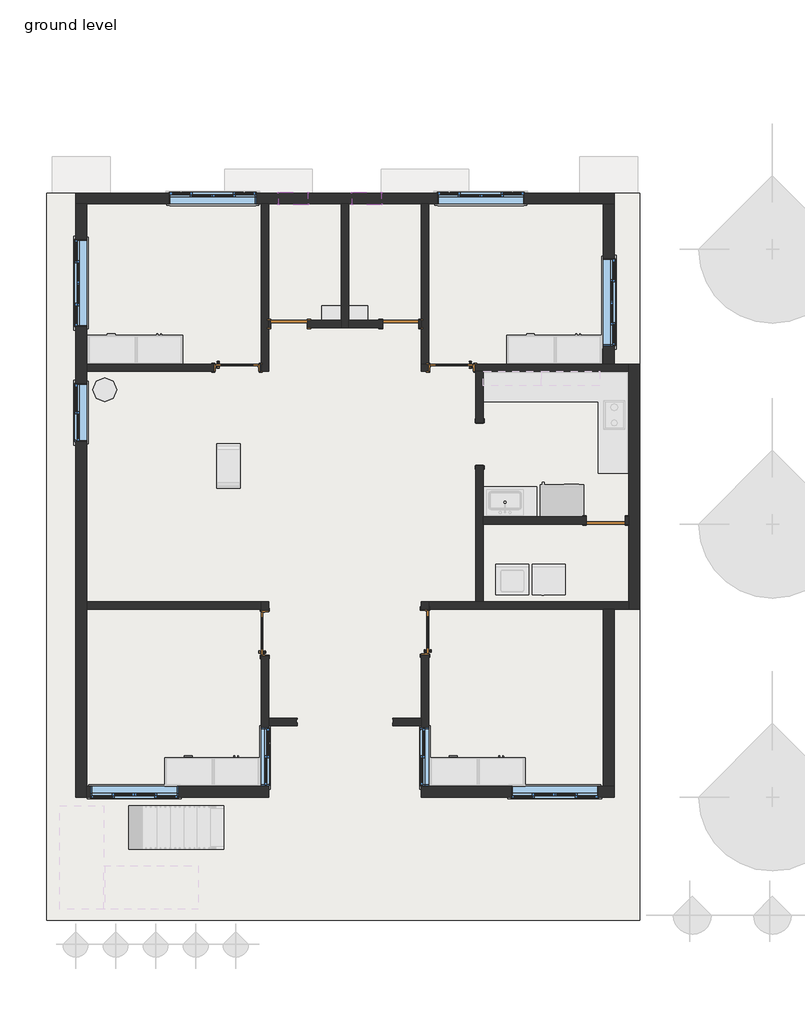
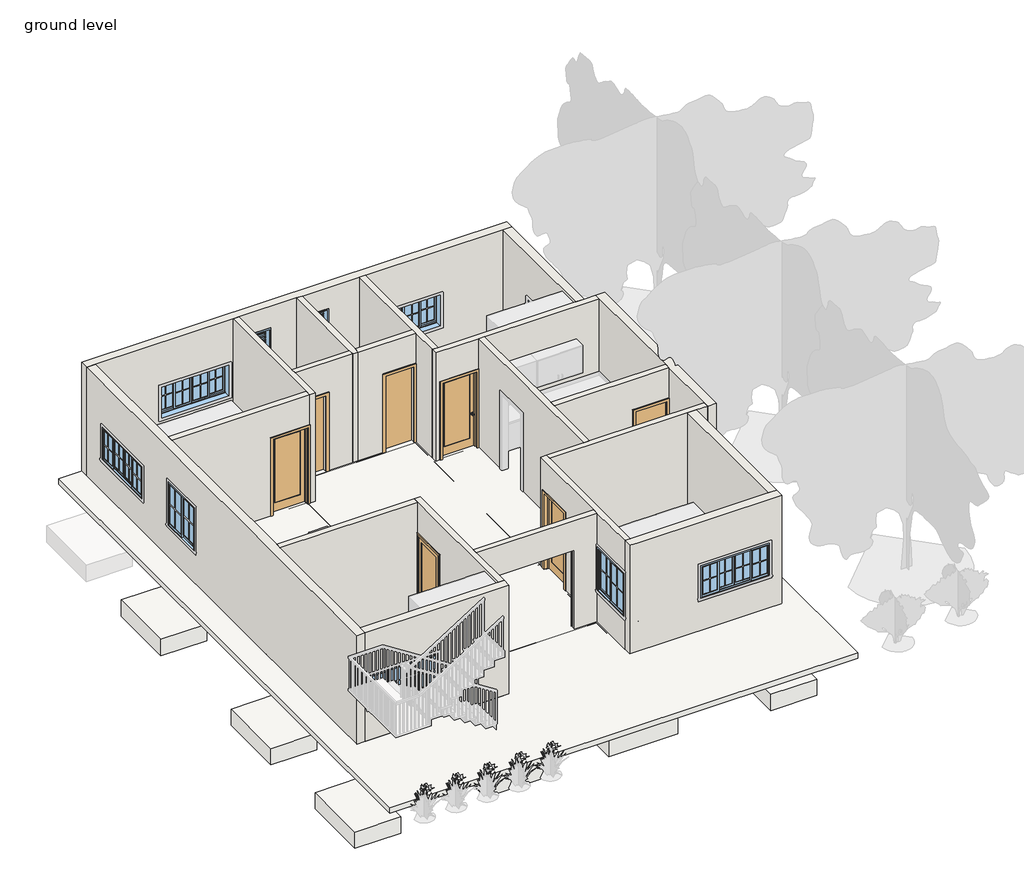
# One storey, part 1 of 4: 21 walls, 11 windows, 10 slabs, 7 beams, 7 doors.
"""IFC4 building model written with IfcOpenShell, lengths in millimetres."""

from ifc_helpers import new_model, si_unit, frame, origin, place, context, project, spatial, polyline, outline, extrude, faceted_brep, transform, mapped, element, save
from components import door_010cc4d9, door_5a860750, door_e2b13fe9, door_a9addea7, door_bb092f7c, window_f2d8fef0, window_c1e3dfc0, window_49fe3060, window_58cce754

model = new_model("IFC4")

# Units and contexts
model_context = context("Model", 3, world=origin())
ifc_project = project(units=[si_unit("LENGTHUNIT", "METRE", prefix="MILLI")], contexts=[model_context])

# Site, building, storey
site = spatial("IfcSite", under=ifc_project)
building = spatial("IfcBuilding", under=site)
storey = spatial("IfcBuildingStorey", under=building, Name="ground level", Elevation=609.6)

# Beams
placement = place(None, origin())
element("IfcBeam", 1, ObjectType="Concrete-Rectangular Beam", at=placement, inside=storey, context=model_context, shape_type="SweptSolid", body=[
    extrude(outline(polyline([(-1593.2124084, 1316.1961804), (-1364.6124084, 1316.1961804), (-1364.6124084, -2163.6038196), (-1593.2124084, -2163.6038196), (-1593.2124084, 1316.1961804)])), frame((0.0, 0.0, 304.8), z_axis=(0.0, 0.0, 1.0), x_axis=(1.0, 0.0, 0.0)), (0.0, 0.0, 1.0), 304.8),
])
element("IfcBeam", 2, ObjectType="Concrete-Rectangular Beam", at=placement, inside=storey, context=model_context, shape_type="Brep", body=[
    faceted_brep([(-1593.2124084, -2430.3038196, 609.6), (-1593.2124084, -2201.7038196, 609.6), (-5212.7124084, -2201.7038196, 609.6), (-5441.3124084, -2201.7038196, 609.6), (-5441.3124084, -2239.8038196, 609.6), (-5174.6124084, -2239.8038196, 609.6), (-5174.6124084, -2430.3038196, 609.6), (-1593.2124084, -2201.7038196, 304.8), (-5212.7124084, -2201.7038196, 304.8), (-5441.3124084, -2201.7038196, 304.8), (-1593.2124084, -2430.3038196, 304.8), (-5174.6124084, -2430.3038196, 304.8), (-5174.6124084, -2239.8038196, 304.8), (-5441.3124084, -2239.8038196, 304.8)], [[[0, 1, 2, 3, 4, 5, 6]], [[1, 7, 8, 9, 3, 2]], [[7, 10, 11, 12, 13, 9, 8]], [[6, 11, 10, 0]], [[0, 10, 7, 1]], [[12, 5, 4, 13]], [[5, 12, 11, 6]], [[3, 9, 13, 4]]]),
])
element("IfcBeam", 3, ObjectType="Concrete-Rectangular Beam", at=placement, inside=storey, context=model_context, shape_type="Brep", body=[
    faceted_brep([(-8756.0124084, -2468.4038196, 609.6), (-8756.0124084, -2239.8038196, 609.6), (-8794.1124084, -2239.8038196, 609.6), (-12413.6124084, -2239.8038196, 609.6), (-12413.6124084, -2468.4038196, 609.6), (-8756.0124084, -2239.8038196, 304.8), (-8794.1124084, -2239.8038196, 304.8), (-12413.6124084, -2239.8038196, 304.8), (-8756.0124084, -2468.4038196, 304.8), (-12413.6124084, -2468.4038196, 304.8)], [[[0, 1, 2, 3, 4]], [[1, 5, 6, 7, 3, 2]], [[5, 8, 9, 7, 6]], [[8, 0, 4, 9]], [[1, 0, 8, 5]], [[4, 3, 7, 9]]]),
])
element("IfcBeam", 4, ObjectType="Concrete-Rectangular Beam", at=placement, inside=storey, context=model_context, shape_type="SweptSolid", body=[
    extrude(outline(polyline([(-12642.2124084, 9875.9961804), (-12413.6124084, 9875.9961804), (-12413.6124084, 6751.7961804), (-12642.2124084, 6751.7961804), (-12642.2124084, 9875.9961804)])), frame((0.0, 0.0, 304.8), z_axis=(0.0, 0.0, 1.0), x_axis=(1.0, 0.0, 0.0)), (0.0, 0.0, 1.0), 304.8),
    extrude(outline(polyline([(-12413.6124084, -2163.6038196), (-12642.2124084, -2163.6038196), (-12642.2124084, 1392.3961804), (-12413.6124084, 1392.3961804), (-12413.6124084, -2163.6038196)])), frame((0.0, 0.0, 304.8), z_axis=(0.0, 0.0, 1.0), x_axis=(1.0, 0.0, 0.0)), (0.0, 0.0, 1.0), 304.8),
    extrude(outline(polyline([(-12413.6124084, 1697.1961804), (-12642.2124084, 1697.1961804), (-12642.2124084, 6446.9961804), (-12413.6124084, 6446.9961804), (-12413.6124084, 1697.1961804)])), frame((0.0, 0.0, 304.8), z_axis=(0.0, 0.0, 1.0), x_axis=(1.0, 0.0, 0.0)), (0.0, 0.0, 1.0), 304.8),
])
element("IfcBeam", 5, ObjectType="Concrete-Rectangular Beam", at=placement, inside=storey, context=model_context, shape_type="Brep", body=[
    faceted_brep([(-843.9124084, 1659.0961804, 609.6), (-843.9124084, 1430.4961804, 609.6), (-843.9124084, 1430.4961804, 304.8), (-843.9124084, 1659.0961804, 304.8), (-5098.4124084, 1659.0961804, 609.6), (-5098.4124084, 1468.5961804, 609.6), (-5403.2124084, 1468.5961804, 609.6), (-5403.2124084, 1659.0961804, 609.6), (-5441.3124084, 1659.0961804, 609.6), (-8565.5124084, 1659.0961804, 609.6), (-8603.6124084, 1659.0961804, 609.6), (-8603.6124084, 1468.5961804, 609.6), (-8908.4124084, 1468.5961804, 609.6), (-8908.4124084, 1659.0961804, 609.6), (-12413.6124084, 1659.0961804, 609.6), (-12413.6124084, 1430.4961804, 609.6), (-8794.1124084, 1430.4961804, 609.6), (-8565.5124084, 1430.4961804, 609.6), (-5441.3124084, 1430.4961804, 609.6), (-5212.7124084, 1430.4961804, 609.6), (-1593.2124084, 1430.4961804, 609.6), (-1593.2124084, 1620.9961804, 609.6), (-1364.6124084, 1620.9961804, 609.6), (-1364.6124084, 1430.4961804, 609.6), (-1364.6124084, 1430.4961804, 304.8), (-1364.6124084, 1620.9961804, 304.8), (-1593.2124084, 1620.9961804, 304.8), (-1593.2124084, 1430.4961804, 304.8), (-5212.7124084, 1430.4961804, 304.8), (-5441.3124084, 1430.4961804, 304.8), (-8565.5124084, 1430.4961804, 304.8), (-8794.1124084, 1430.4961804, 304.8), (-12413.6124084, 1430.4961804, 304.8), (-12413.6124084, 1659.0961804, 304.8), (-8908.4124084, 1659.0961804, 304.8), (-8908.4124084, 1468.5961804, 304.8), (-8603.6124084, 1468.5961804, 304.8), (-8603.6124084, 1659.0961804, 304.8), (-8565.5124084, 1659.0961804, 304.8), (-5441.3124084, 1659.0961804, 304.8), (-5403.2124084, 1659.0961804, 304.8), (-5403.2124084, 1468.5961804, 304.8), (-5098.4124084, 1468.5961804, 304.8), (-5098.4124084, 1659.0961804, 304.8)], [[[0, 1, 2, 3]], [[1, 0, 4, 5, 6, 7, 8, 9, 10, 11, 12, 13, 14, 15, 16, 17, 18, 19, 20, 21, 22, 23]], [[2, 1, 23, 24]], [[3, 2, 24, 25, 26, 27, 28, 29, 30, 31, 32, 33, 34, 35, 36, 37, 38, 39, 40, 41, 42, 43]], [[0, 3, 43, 4]], [[15, 14, 33, 32]], [[22, 25, 24, 23]], [[26, 21, 20, 27]], [[21, 26, 25, 22]], [[36, 11, 10, 37]], [[11, 36, 35, 12]], [[12, 35, 34, 13]], [[42, 5, 4, 43]], [[5, 42, 41, 6]], [[6, 41, 40, 7]], [[15, 32, 31, 30, 29, 28, 27, 20, 19, 18, 17, 16]], [[33, 14, 13, 34]], [[37, 10, 9, 8, 7, 40, 39, 38]]]),
])
element("IfcBeam", 6, ObjectType="Concrete-Rectangular Beam", at=placement, inside=storey, context=model_context, shape_type="Brep", body=[
    faceted_brep([(-8794.1124084, -2239.8038196, 609.6), (-8756.0124084, -2239.8038196, 609.6), (-8565.5124084, -2239.8038196, 609.6), (-8565.5124084, -1007.9038196, 609.6), (-8565.5124084, -779.3038196, 609.6), (-8565.5124084, 1430.4961804, 609.6), (-8794.1124084, 1430.4961804, 609.6), (-8794.1124084, -2239.8038196, 304.8), (-8794.1124084, 1430.4961804, 304.8), (-8565.5124084, -2239.8038196, 304.8), (-8756.0124084, -2239.8038196, 304.8), (-8565.5124084, 1430.4961804, 304.8), (-8565.5124084, -779.3038196, 304.8), (-8565.5124084, -1007.9038196, 304.8)], [[[0, 1, 2, 3, 4, 5, 6]], [[7, 0, 6, 8]], [[9, 10, 7, 8, 11, 12, 13]], [[2, 9, 13, 12, 11, 5, 4, 3]], [[2, 1, 0, 7, 10, 9]], [[6, 5, 11, 8]]]),
    faceted_brep([(-8794.1124084, 9914.0961804, 609.6), (-8565.5124084, 9914.0961804, 609.6), (-8565.5124084, 9914.0961804, 304.8), (-8794.1124084, 9914.0961804, 304.8), (-8756.0124084, 6751.7961804, 304.8), (-8756.0124084, 6751.7961804, 609.6), (-8756.0124084, 6713.6961804, 609.6), (-8756.0124084, 6713.6961804, 304.8), (-8565.5124084, 6751.7961804, 304.8), (-8565.5124084, 6751.7961804, 609.6), (-8794.1124084, 6713.6961804, 609.6), (-8794.1124084, 6713.6961804, 304.8), (-8565.5124084, 7323.2961804, 609.6), (-8565.5124084, 7551.8961804, 609.6), (-8565.5124084, 7551.8961804, 304.8), (-8565.5124084, 7323.2961804, 304.8)], [[[0, 1, 2, 3]], [[4, 5, 6, 7]], [[5, 4, 8, 9]], [[6, 10, 11, 7]], [[1, 0, 10, 6, 5, 9, 12, 13]], [[3, 2, 14, 15, 8, 4, 7, 11]], [[2, 1, 13, 12, 9, 8, 15, 14]], [[0, 3, 11, 10]]]),
    faceted_brep([(-8756.0124084, 6446.9961804, 304.8), (-8756.0124084, 6446.9961804, 609.6), (-8565.5124084, 6446.9961804, 609.6), (-8565.5124084, 6446.9961804, 304.8), (-8603.6124084, 1697.1961804, 304.8), (-8603.6124084, 1697.1961804, 609.6), (-8794.1124084, 1697.1961804, 609.6), (-8794.1124084, 1697.1961804, 304.8), (-8603.6124084, 1659.0961804, 304.8), (-8603.6124084, 1659.0961804, 609.6), (-8794.1124084, 6485.0961804, 609.6), (-8756.0124084, 6485.0961804, 609.6), (-8756.0124084, 6485.0961804, 304.8), (-8794.1124084, 6485.0961804, 304.8), (-8565.5124084, 1659.0961804, 609.6), (-8565.5124084, 1659.0961804, 304.8)], [[[0, 1, 2, 3]], [[4, 5, 6, 7]], [[5, 4, 8, 9]], [[10, 11, 12, 13]], [[14, 9, 8, 15]], [[7, 6, 10, 13]], [[1, 0, 12, 11]], [[11, 10, 6, 5, 9, 14, 2, 1]], [[13, 12, 0, 3, 15, 8, 4, 7]], [[3, 2, 14, 15]]]),
])
element("IfcBeam", 7, ObjectType="Concrete-Rectangular Beam", at=placement, inside=storey, context=model_context, shape_type="SweptSolid", body=[
    extrude(outline(polyline([(-5441.3124084, -779.3038196), (-5441.3124084, -1007.9038196), (-8565.5124084, -1007.9038196), (-8565.5124084, -779.3038196), (-5441.3124084, -779.3038196)])), frame((0.0, 0.0, 304.8), z_axis=(0.0, 0.0, 1.0), x_axis=(1.0, 0.0, 0.0)), (0.0, 0.0, 1.0), 304.8),
])

# Doors
door_shape = door_010cc4d9(model_context)
element("IfcDoor", 8, ObjectType="Door-Interior-Single-1_Panel-Wood : 36\" x 84\"", at=placement, inside=storey, context=model_context, shape_type="MappedRepresentation", body=[
    mapped(door_shape, transform((-9264.0124084, 6526.3711804, 609.6), x_axis=(1.0, 0.0, 0.0), y_axis=(0.0, 1.0, 0.0), z_axis=(0.0, 0.0, 1.0))),
])
element("IfcDoor", 9, ObjectType="Door-Interior-Single-1_Panel-Wood : 36\" x 84\"", at=placement, inside=storey, context=model_context, shape_type="MappedRepresentation", body=[
    mapped(door_shape, transform((-8682.9874084, 960.5961804, 609.6), x_axis=(0.0, 1.0, 0.0), y_axis=(-1.0, 0.0, 0.0), z_axis=(0.0, 0.0, 1.0))),
])
door_2_shape = door_5a860750(model_context)
element("IfcDoor", 10, ObjectType="Door-Interior-Single-1_Panel-Wood : 36\" x 84\"", at=placement, inside=storey, context=model_context, shape_type="MappedRepresentation", body=[
    mapped(door_2_shape, transform((-4768.2124084, 6526.3711804, 609.6), x_axis=(-1.0, 0.0, 0.0), y_axis=(0.0, -1.0, 0.0), z_axis=(0.0, 0.0, 1.0))),
])
element("IfcDoor", 11, ObjectType="Door-Interior-Single-1_Panel-Wood : 36\" x 84\"", at=placement, inside=storey, context=model_context, shape_type="MappedRepresentation", body=[
    mapped(door_2_shape, transform((-5323.8374084, 985.9961804, 609.6), x_axis=(0.0, 1.0, 0.0), y_axis=(-1.0, 0.0, 0.0), z_axis=(0.0, 0.0, 1.0))),
])
door_3_shape = door_e2b13fe9(model_context)
element("IfcDoor", 12, ObjectType="Single-Flush : 30\" x 84\"", at=placement, inside=storey, context=model_context, shape_type="MappedRepresentation", body=[
    mapped(door_3_shape, transform((-8171.8124084, 7437.5961804, 609.6), x_axis=(-1.0, 0.0, 0.0), y_axis=(0.0, -1.0, 0.0), z_axis=(0.0, 0.0, 1.0))),
])
door_4_shape = door_a9addea7(model_context)
element("IfcDoor", 13, ObjectType="Single-Flush : 30\" x 84\"", at=placement, inside=storey, context=model_context, shape_type="MappedRepresentation", body=[
    mapped(door_4_shape, transform((-5835.0124084, 7437.5961804, 609.6), x_axis=(1.0, 0.0, 0.0), y_axis=(0.0, 1.0, 0.0), z_axis=(0.0, 0.0, 1.0))),
])
door_5_shape = door_bb092f7c(model_context)
element("IfcDoor", 14, ObjectType="Single-Flush : 32\" x 84\"", at=placement, inside=storey, context=model_context, shape_type="MappedRepresentation", body=[
    mapped(door_5_shape, transform((-1542.4124084, 3322.7961804, 609.6), x_axis=(1.0, 0.0, 0.0), y_axis=(0.0, 1.0, 0.0), z_axis=(0.0, 0.0, 1.0))),
])

# Slabs
element("IfcSlab", 15, ObjectType="Footing-Rectangular : 72\" x 48\" x 18\"", at=placement, inside=storey, context=model_context, shape_type="SweptSolid", body=[
    extrude(outline(polyline([(-869.3124084, -1401.6038196), (-869.3124084, -3230.4038196), (-2088.5124084, -3230.4038196), (-2088.5124084, -1401.6038196), (-869.3124084, -1401.6038196)])), frame((0.0, 0.0, -1676.4), z_axis=(0.0, 0.0, 1.0), x_axis=(1.0, 0.0, 0.0)), (0.0, 0.0, 1.0), 457.2),
])
element("IfcSlab", 16, ObjectType="Footing-Rectangular : 72\" x 48\" x 18\"", at=placement, inside=storey, context=model_context, shape_type="SweptSolid", body=[
    extrude(outline(polyline([(-6241.4124084, -1744.5038196), (-4412.6124084, -1744.5038196), (-4412.6124084, -2963.7038196), (-6241.4124084, -2963.7038196), (-6241.4124084, -1744.5038196)])), frame((0.0, 0.0, -1676.4), z_axis=(0.0, 0.0, 1.0), x_axis=(1.0, 0.0, 0.0)), (0.0, 0.0, 1.0), 457.2),
])
element("IfcSlab", 17, ObjectType="Footing-Rectangular : 72\" x 48\" x 18\"", at=placement, inside=storey, context=model_context, shape_type="SweptSolid", body=[
    extrude(outline(polyline([(-9518.0124084, -1744.5038196), (-7689.2124084, -1744.5038196), (-7689.2124084, -2963.7038196), (-9518.0124084, -2963.7038196), (-9518.0124084, -1744.5038196)])), frame((0.0, 0.0, -1676.4), z_axis=(0.0, 0.0, 1.0), x_axis=(1.0, 0.0, 0.0)), (0.0, 0.0, 1.0), 457.2),
])
element("IfcSlab", 18, ObjectType="Footing-Rectangular : 72\" x 48\" x 18\"", at=placement, inside=storey, context=model_context, shape_type="SweptSolid", body=[
    extrude(outline(polyline([(-13137.5124084, -3230.4038196), (-13137.5124084, -1401.6038196), (-11918.3124084, -1401.6038196), (-11918.3124084, -3230.4038196), (-13137.5124084, -3230.4038196)])), frame((0.0, 0.0, -1676.4), z_axis=(0.0, 0.0, 1.0), x_axis=(1.0, 0.0, 0.0)), (0.0, 0.0, 1.0), 457.2),
])
element("IfcSlab", 19, ObjectType="Footing-Rectangular : 72\" x 48\" x 18\"", at=placement, inside=storey, context=model_context, shape_type="SweptSolid", body=[
    extrude(outline(polyline([(-11918.3124084, 2459.1961804), (-11918.3124084, 630.3961804), (-13137.5124084, 630.3961804), (-13137.5124084, 2459.1961804), (-11918.3124084, 2459.1961804)])), frame((0.0, 0.0, -1676.4), z_axis=(0.0, 0.0, 1.0), x_axis=(1.0, 0.0, 0.0)), (0.0, 0.0, 1.0), 457.2),
])
element("IfcSlab", 20, ObjectType="Footing-Rectangular : 72\" x 48\" x 18\"", at=placement, inside=storey, context=model_context, shape_type="SweptSolid", body=[
    extrude(outline(polyline([(-11918.3124084, 7513.7961804), (-11918.3124084, 5684.9961804), (-13137.5124084, 5684.9961804), (-13137.5124084, 7513.7961804), (-11918.3124084, 7513.7961804)])), frame((0.0, 0.0, -1676.4), z_axis=(0.0, 0.0, 1.0), x_axis=(1.0, 0.0, 0.0)), (0.0, 0.0, 1.0), 457.2),
])
element("IfcSlab", 21, ObjectType="Footing-Rectangular : 72\" x 48\" x 18\"", at=placement, inside=storey, context=model_context, shape_type="SweptSolid", body=[
    extrude(outline(polyline([(-8032.1124084, 7513.7961804), (-8032.1124084, 5684.9961804), (-9251.3124084, 5684.9961804), (-9251.3124084, 7513.7961804), (-8032.1124084, 7513.7961804)])), frame((0.0, 0.0, -1676.4), z_axis=(0.0, 0.0, 1.0), x_axis=(1.0, 0.0, 0.0)), (0.0, 0.0, 1.0), 457.2),
])
element("IfcSlab", 22, ObjectType="Footing-Rectangular : 72\" x 48\" x 18\"", at=placement, inside=storey, context=model_context, shape_type="SweptSolid", body=[
    extrude(outline(polyline([(-9670.4124084, 2192.4961804), (-7841.6124084, 2192.4961804), (-7841.6124084, 973.2961804), (-9670.4124084, 973.2961804), (-9670.4124084, 2192.4961804)])), frame((0.0, 0.0, -1676.4), z_axis=(0.0, 0.0, 1.0), x_axis=(1.0, 0.0, 0.0)), (0.0, 0.0, 1.0), 457.2),
])
element("IfcSlab", 23, ObjectType="Footing-Rectangular : 72\" x 48\" x 18\"", at=placement, inside=storey, context=model_context, shape_type="SweptSolid", body=[
    extrude(outline(polyline([(-6165.2124084, 2192.4961804), (-4336.4124084, 2192.4961804), (-4336.4124084, 973.2961804), (-6165.2124084, 973.2961804), (-6165.2124084, 2192.4961804)])), frame((0.0, 0.0, -1676.4), z_axis=(0.0, 0.0, 1.0), x_axis=(1.0, 0.0, 0.0)), (0.0, 0.0, 1.0), 457.2),
])
element("IfcSlab", 24, ObjectType="Generic - 6\"", at=placement, inside=storey, context=model_context, shape_type="SweptSolid", body=[
    extrude(outline(polyline([(-831.2124084, 10180.7961804), (-831.2124084, -5046.5038196), (-13251.8124084, -5046.5038196), (-13251.8124084, 10180.7961804), (-831.2124084, 10180.7961804)])), frame((0.0, 0.0, 457.2), z_axis=(0.0, 0.0, 1.0), x_axis=(1.0, 0.0, 0.0)), (0.0, 0.0, 1.0), 152.4),
])

# Walls
element("IfcWall", 25, ObjectType="Generic - 6\"", at=placement, inside=storey, context=model_context, shape_type="Brep", body=[
    faceted_brep([(-8756.0124084, 9952.1961804, 609.6), (-8756.0124084, 6599.3961804, 609.6), (-8756.0124084, 6446.9961804, 609.6), (-8756.0124084, 6446.9961804, 3657.6), (-8756.0124084, 6599.3961804, 3657.6), (-8756.0124084, 9952.1961804, 3657.6), (-8603.6124084, 9952.1961804, 609.6), (-8603.6124084, 9952.1961804, 3657.6), (-8603.6124084, 7513.7961804, 3657.6), (-8603.6124084, 7361.3961804, 3657.6), (-8603.6124084, 6446.9961804, 3657.6), (-8603.6124084, 6446.9961804, 609.6), (-8603.6124084, 7361.3961804, 609.6), (-8603.6124084, 7513.7961804, 609.6)], [[[0, 1, 2, 3, 4, 5]], [[6, 7, 8, 9, 10, 11, 12, 13]], [[2, 1, 0, 6, 13, 12, 11]], [[0, 5, 7, 6]], [[3, 2, 11, 10]], [[5, 4, 3, 10, 9, 8, 7]]]),
])
element("IfcWall", 26, ObjectType="Generic - 6\"", at=placement, inside=storey, context=model_context, shape_type="SweptSolid", body=[
    extrude(outline(polyline([(609.6, -8756.0124084), (3657.6, -8756.0124084), (3657.6, -12413.6124084), (609.6, -12413.6124084), (609.6, -9746.6124084), (2768.6, -9746.6124084), (2768.6, -8781.4124084), (609.6, -8781.4124084), (609.6, -8756.0124084)])), frame((0.0, 6446.9961804, 0.0), z_axis=(0.0, 1.0, 0.0), x_axis=(0.0, 0.0, 1.0)), (0.0, 0.0, 1.0), 152.4),
])
element("IfcWall", 27, ObjectType="Generic - 6\"", at=placement, inside=storey, context=model_context, shape_type="Brep", body=[
    faceted_brep([(-7079.6124084, 9952.1961804, 609.6), (-7079.6124084, 7513.7961804, 609.6), (-7079.6124084, 7361.3961804, 609.6), (-7079.6124084, 7361.3961804, 3657.6), (-7079.6124084, 7513.7961804, 3657.6), (-7079.6124084, 9952.1961804, 3657.6), (-6927.2124084, 9952.1961804, 609.6), (-6927.2124084, 9952.1961804, 3657.6), (-6927.2124084, 7513.7961804, 3657.6), (-6927.2124084, 7361.3961804, 3657.6), (-6927.2124084, 7361.3961804, 609.6), (-6927.2124084, 7513.7961804, 609.6)], [[[0, 1, 2, 3, 4, 5]], [[6, 7, 8, 9, 10, 11]], [[2, 1, 0, 6, 11, 10]], [[0, 5, 7, 6]], [[3, 2, 10, 9]], [[5, 4, 3, 9, 8, 7]]]),
])
element("IfcWall", 28, ObjectType="Generic - 6\"", at=placement, inside=storey, context=model_context, shape_type="SweptSolid", body=[
    extrude(outline(polyline([(609.6, -7079.6124084), (3657.6, -7079.6124084), (3657.6, -8603.6124084), (609.6, -8603.6124084), (609.6, -8552.8124084), (2743.2, -8552.8124084), (2743.2, -7790.8124084), (609.6, -7790.8124084), (609.6, -7079.6124084)])), frame((0.0, 7361.3961804, 0.0), z_axis=(0.0, 1.0, 0.0), x_axis=(0.0, 0.0, 1.0)), (0.0, 0.0, 1.0), 152.4),
])
element("IfcWall", 29, ObjectType="Generic - 6\"", at=placement, inside=storey, context=model_context, shape_type="SweptSolid", body=[
    extrude(outline(polyline([(3657.6, -6927.2124084), (609.6, -6927.2124084), (609.6, -6216.0124084), (2743.2, -6216.0124084), (2743.2, -5454.0124084), (609.6, -5454.0124084), (609.6, -5403.2124084), (3657.6, -5403.2124084), (3657.6, -6927.2124084)])), frame((0.0, 7361.3961804, 0.0), z_axis=(0.0, 1.0, 0.0), x_axis=(0.0, 0.0, 1.0)), (0.0, 0.0, 1.0), 152.4),
])
element("IfcWall", 30, ObjectType="Generic - 6\"", at=placement, inside=storey, context=model_context, shape_type="Brep", body=[
    faceted_brep([(-5250.8124084, 6599.3961804, 609.6), (-5250.8124084, 9952.1961804, 609.6), (-5250.8124084, 9952.1961804, 3657.6), (-5250.8124084, 6599.3961804, 3657.6), (-5403.2124084, 6599.3961804, 609.6), (-5403.2124084, 6599.3961804, 3657.6), (-5403.2124084, 7361.3961804, 3657.6), (-5403.2124084, 7513.7961804, 3657.6), (-5403.2124084, 9952.1961804, 3657.6), (-5403.2124084, 9952.1961804, 609.6), (-5403.2124084, 7513.7961804, 609.6), (-5403.2124084, 7361.3961804, 609.6)], [[[0, 1, 2, 3]], [[4, 5, 6, 7, 8, 9, 10, 11]], [[1, 0, 4, 11, 10, 9]], [[2, 1, 9, 8]], [[0, 3, 5, 4]], [[3, 2, 8, 7, 6, 5]]]),
])
element("IfcWall", 31, ObjectType="Generic - 6\"", at=placement, inside=storey, context=model_context, shape_type="Brep", body=[
    faceted_brep([(-5403.2124084, 6599.3961804, 609.6), (-5403.2124084, 6599.3961804, 3657.6), (-5250.8124084, 6599.3961804, 3657.6), (-1593.2124084, 6599.3961804, 3657.6), (-1364.6124084, 6599.3961804, 3657.6), (-1059.8124084, 6599.3961804, 3657.6), (-1059.8124084, 6599.3961804, 609.6), (-1364.6124084, 6599.3961804, 609.6), (-1593.2124084, 6599.3961804, 609.6), (-4285.6124084, 6599.3961804, 609.6), (-4285.6124084, 6599.3961804, 2768.6), (-5250.8124084, 6599.3961804, 2768.6), (-5250.8124084, 6599.3961804, 609.6), (-1059.8124084, 6446.9961804, 3657.6), (-4107.8124084, 6446.9961804, 3657.6), (-4260.2124084, 6446.9961804, 3657.6), (-5403.2124084, 6446.9961804, 3657.6), (-5403.2124084, 6446.9961804, 609.6), (-5250.8124084, 6446.9961804, 609.6), (-5250.8124084, 6446.9961804, 2768.6), (-4285.6124084, 6446.9961804, 2768.6), (-4285.6124084, 6446.9961804, 609.6), (-4260.2124084, 6446.9961804, 609.6), (-4107.8124084, 6446.9961804, 609.6), (-1059.8124084, 6446.9961804, 609.6)], [[[0, 1, 2, 3, 4, 5, 6, 7, 8, 9, 10, 11, 12]], [[13, 14, 15, 16, 17, 18, 19, 20, 21, 22, 23, 24]], [[17, 0, 12, 18]], [[6, 24, 23, 22, 21, 9, 8, 7]], [[1, 0, 17, 16]], [[6, 5, 13, 24]], [[11, 19, 18, 12]], [[19, 11, 10, 20]], [[20, 10, 9, 21]], [[16, 15, 14, 13, 5, 4, 3, 2, 1]]]),
])
element("IfcWall", 32, ObjectType="Generic - 6\"", at=placement, inside=storey, context=model_context, shape_type="SweptSolid", body=[
    extrude(outline(polyline([(-8756.0124084, 1468.5961804), (-12413.6124084, 1468.5961804), (-12413.6124084, 1620.9961804), (-8756.0124084, 1620.9961804), (-8756.0124084, 1468.5961804)])), frame((0.0, 0.0, 609.6), z_axis=(0.0, 0.0, 1.0), x_axis=(1.0, 0.0, 0.0)), (0.0, 0.0, 1.0), 3048.0),
])
element("IfcWall", 33, ObjectType="Generic - 6\"", at=placement, inside=storey, context=model_context, shape_type="Brep", body=[
    faceted_brep([(-5403.2124084, 1620.9961804, 3657.6), (-5403.2124084, 1620.9961804, 609.6), (-5403.2124084, 1468.5961804, 609.6), (-5403.2124084, 1468.5961804, 2768.6), (-5403.2124084, 503.3961804, 2768.6), (-5403.2124084, 503.3961804, 609.6), (-5403.2124084, -817.4038196, 609.6), (-5403.2124084, -969.8038196, 609.6), (-5403.2124084, -2239.8038196, 609.6), (-5403.2124084, -2239.8038196, 3657.6), (-5403.2124084, -969.8038196, 3657.6), (-5403.2124084, -817.4038196, 3657.6), (-5403.2124084, -1014.2538196, 1524.0), (-5403.2124084, -1014.2538196, 2743.2), (-5403.2124084, -2233.4538196, 2743.2), (-5403.2124084, -2233.4538196, 1524.0), (-5250.8124084, 1620.9961804, 609.6), (-5250.8124084, 1620.9961804, 3657.6), (-5250.8124084, 1468.5961804, 3657.6), (-5250.8124084, -2239.8038196, 3657.6), (-5250.8124084, -2239.8038196, 609.6), (-5250.8124084, 503.3961804, 609.6), (-5250.8124084, 503.3961804, 2768.6), (-5250.8124084, 1468.5961804, 2768.6), (-5250.8124084, 1468.5961804, 609.6), (-5250.8124084, -1014.2538196, 2743.2), (-5250.8124084, -1014.2538196, 1524.0), (-5250.8124084, -2233.4538196, 1524.0), (-5250.8124084, -2233.4538196, 2743.2)], [[[0, 1, 2, 3, 4, 5, 6, 7, 8, 9, 10, 11], [12, 13, 14, 15]], [[16, 17, 18, 19, 20, 21, 22, 23, 24], [25, 26, 27, 28]], [[1, 16, 24, 2]], [[8, 7, 6, 5, 21, 20]], [[1, 0, 17, 16]], [[23, 3, 2, 24]], [[3, 23, 22, 4]], [[4, 22, 21, 5]], [[25, 13, 12, 26]], [[26, 12, 15, 27]], [[27, 15, 14, 28]], [[13, 25, 28, 14]], [[0, 11, 10, 9, 19, 18, 17]], [[9, 8, 20, 19]]]),
])
element("IfcWall", 34, ObjectType="Generic - 6\"", at=placement, inside=storey, context=model_context, shape_type="Brep", body=[
    faceted_brep([(-8756.0124084, 1620.9961804, 609.6), (-8756.0124084, 1468.5961804, 609.6), (-8756.0124084, 1443.1961804, 609.6), (-8756.0124084, 1443.1961804, 2768.6), (-8756.0124084, 477.9961804, 2768.6), (-8756.0124084, 477.9961804, 609.6), (-8756.0124084, -2239.8038196, 609.6), (-8756.0124084, -2239.8038196, 3657.6), (-8756.0124084, 1468.5961804, 3657.6), (-8756.0124084, 1620.9961804, 3657.6), (-8756.0124084, -2233.4538196, 2743.2), (-8756.0124084, -2233.4538196, 1524.0), (-8756.0124084, -1014.2538196, 1524.0), (-8756.0124084, -1014.2538196, 2743.2), (-8603.6124084, 1443.1961804, 609.6), (-8603.6124084, 1620.9961804, 609.6), (-8603.6124084, 1620.9961804, 3657.6), (-8603.6124084, -817.4038196, 3657.6), (-8603.6124084, -969.8038196, 3657.6), (-8603.6124084, -2239.8038196, 3657.6), (-8603.6124084, -2239.8038196, 609.6), (-8603.6124084, -969.8038196, 609.6), (-8603.6124084, -817.4038196, 609.6), (-8603.6124084, 477.9961804, 609.6), (-8603.6124084, 477.9961804, 2768.6), (-8603.6124084, 1443.1961804, 2768.6), (-8603.6124084, -2233.4538196, 1524.0), (-8603.6124084, -2233.4538196, 2743.2), (-8603.6124084, -1014.2538196, 2743.2), (-8603.6124084, -1014.2538196, 1524.0)], [[[0, 1, 2, 3, 4, 5, 6, 7, 8, 9], [10, 11, 12, 13]], [[14, 15, 16, 17, 18, 19, 20, 21, 22, 23, 24, 25], [26, 27, 28, 29]], [[6, 5, 23, 22, 21, 20]], [[2, 1, 0, 15, 14]], [[25, 3, 2, 14]], [[3, 25, 24, 4]], [[4, 24, 23, 5]], [[0, 9, 16, 15]], [[10, 27, 26, 11]], [[11, 26, 29, 12]], [[12, 29, 28, 13]], [[27, 10, 13, 28]], [[9, 8, 7, 19, 18, 17, 16]], [[7, 6, 20, 19]]]),
])
element("IfcWall", 35, ObjectType="Generic - 6\"", at=placement, inside=storey, context=model_context, shape_type="Brep", body=[
    faceted_brep([(-4260.2124084, 6446.9961804, 3657.6), (-4260.2124084, 6446.9961804, 609.6), (-4260.2124084, 5380.1961804, 609.6), (-4260.2124084, 5380.1961804, 2743.2), (-4260.2124084, 4465.7961804, 2743.2), (-4260.2124084, 4465.7961804, 609.6), (-4260.2124084, 1620.9961804, 609.6), (-4260.2124084, 1620.9961804, 3657.6), (-4107.8124084, 6446.9961804, 609.6), (-4107.8124084, 6446.9961804, 3657.6), (-4107.8124084, 3398.9961804, 3657.6), (-4107.8124084, 3246.5961804, 3657.6), (-4107.8124084, 1620.9961804, 3657.6), (-4107.8124084, 1620.9961804, 609.6), (-4107.8124084, 3246.5961804, 609.6), (-4107.8124084, 3398.9961804, 609.6), (-4107.8124084, 4465.7961804, 609.6), (-4107.8124084, 4465.7961804, 2743.2), (-4107.8124084, 5380.1961804, 2743.2), (-4107.8124084, 5380.1961804, 609.6)], [[[0, 1, 2, 3, 4, 5, 6, 7]], [[8, 9, 10, 11, 12, 13, 14, 15, 16, 17, 18, 19]], [[1, 8, 19, 2]], [[13, 6, 5, 16, 15, 14]], [[1, 0, 9, 8]], [[7, 6, 13, 12]], [[4, 17, 16, 5]], [[18, 3, 2, 19]], [[17, 4, 3, 18]], [[0, 7, 12, 11, 10, 9]]]),
])
element("IfcWall", 36, ObjectType="Generic - 6\"", at=placement, inside=storey, context=model_context, shape_type="SweptSolid", body=[
    extrude(outline(polyline([(3657.6, -4107.8124084), (609.6, -4107.8124084), (609.6, -1948.8124084), (2743.2, -1948.8124084), (2743.2, -1136.0124084), (609.6, -1136.0124084), (609.6, -1059.8124084), (3657.6, -1059.8124084), (3657.6, -4107.8124084)])), frame((0.0, 3246.5961804, 0.0), z_axis=(0.0, 1.0, 0.0), x_axis=(0.0, 0.0, 1.0)), (0.0, 0.0, 1.0), 152.4),
])
element("IfcWall", 37, ObjectType="Generic - 6\"", at=placement, inside=storey, context=model_context, shape_type="Brep", body=[
    faceted_brep([(-5250.8124084, 1468.5961804, 609.6), (-1593.2124084, 1468.5961804, 609.6), (-1364.6124084, 1468.5961804, 609.6), (-1059.8124084, 1468.5961804, 609.6), (-1059.8124084, 1468.5961804, 3657.6), (-1364.6124084, 1468.5961804, 3657.6), (-1593.2124084, 1468.5961804, 3657.6), (-5250.8124084, 1468.5961804, 3657.6), (-5250.8124084, 1620.9961804, 609.6), (-5250.8124084, 1620.9961804, 3657.6), (-4260.2124084, 1620.9961804, 3657.6), (-4107.8124084, 1620.9961804, 3657.6), (-1059.8124084, 1620.9961804, 3657.6), (-1059.8124084, 1620.9961804, 609.6), (-4107.8124084, 1620.9961804, 609.6), (-4260.2124084, 1620.9961804, 609.6)], [[[0, 1, 2, 3, 4, 5, 6, 7]], [[8, 9, 10, 11, 12, 13, 14, 15]], [[3, 2, 1, 0, 8, 15, 14, 13]], [[4, 3, 13, 12]], [[0, 7, 9, 8]], [[7, 6, 5, 4, 12, 11, 10, 9]]]),
])
element("IfcWall", 38, ObjectType="Generic - 6\"", at=placement, inside=storey, context=model_context, shape_type="Brep", body=[
    faceted_brep([(-5403.2124084, -969.8038196, 609.6), (-5403.2124084, -969.8038196, 3657.6), (-8603.6124084, -969.8038196, 3657.6), (-8603.6124084, -969.8038196, 609.6), (-8003.4124084, -969.8038196, 609.6), (-8003.4124084, -969.8038196, 2818.6), (-6003.4124084, -969.8038196, 2818.6), (-6003.4124084, -969.8038196, 609.6), (-5403.2124084, -817.4038196, 3657.6), (-5403.2124084, -817.4038196, 609.6), (-6003.4124084, -817.4038196, 609.6), (-6003.4124084, -817.4038196, 2818.6), (-8003.4124084, -817.4038196, 2818.6), (-8003.4124084, -817.4038196, 609.6), (-8603.6124084, -817.4038196, 609.6), (-8603.6124084, -817.4038196, 3657.6), (-8003.4124084, -837.4038196, 609.6), (-8018.4124084, -837.4038196, 609.6), (-8018.4124084, -907.4038196, 609.6), (-8003.4124084, -907.4038196, 609.6), (-6003.4124084, -907.4038196, 609.6), (-5988.4124084, -907.4038196, 609.6), (-5988.4124084, -837.4038196, 609.6), (-6003.4124084, -837.4038196, 609.6), (-6003.4124084, -837.4038196, 2818.6), (-8003.4124084, -837.4038196, 2818.6), (-8003.4124084, -907.4038196, 2818.6), (-6003.4124084, -907.4038196, 2818.6), (-8018.4124084, -907.4038196, 2833.6), (-5988.4124084, -907.4038196, 2833.6), (-5988.4124084, -837.4038196, 2833.6), (-8018.4124084, -837.4038196, 2833.6)], [[[0, 1, 2, 3, 4, 5, 6, 7]], [[8, 9, 10, 11, 12, 13, 14, 15]], [[3, 14, 13, 16, 17, 18, 19, 4]], [[9, 0, 7, 20, 21, 22, 23, 10]], [[1, 0, 9, 8]], [[3, 2, 15, 14]], [[24, 25, 12, 11]], [[26, 27, 6, 5]], [[19, 26, 5, 4]], [[27, 20, 7, 6]], [[27, 26, 19, 18, 28, 29, 21, 20]], [[21, 29, 30, 22]], [[25, 24, 23, 22, 30, 31, 17, 16]], [[23, 24, 11, 10]], [[25, 16, 13, 12]], [[28, 18, 17, 31]], [[29, 28, 31, 30]], [[2, 1, 8, 15]]]),
])
element("IfcWall", 39, ObjectType="Generic - 9\"", at=placement, inside=storey, context=model_context, shape_type="Brep", body=[
    faceted_brep([(-12642.2124084, 9952.1961804, 609.6), (-12413.6124084, 9952.1961804, 609.6), (-8756.0124084, 9952.1961804, 609.6), (-8603.6124084, 9952.1961804, 609.6), (-7079.6124084, 9952.1961804, 609.6), (-6927.2124084, 9952.1961804, 609.6), (-5403.2124084, 9952.1961804, 609.6), (-5250.8124084, 9952.1961804, 609.6), (-1593.2124084, 9952.1961804, 609.6), (-1364.6124084, 9952.1961804, 609.6), (-1364.6124084, 9952.1961804, 3657.6), (-1593.2124084, 9952.1961804, 3657.6), (-5250.8124084, 9952.1961804, 3657.6), (-5403.2124084, 9952.1961804, 3657.6), (-6927.2124084, 9952.1961804, 3657.6), (-7079.6124084, 9952.1961804, 3657.6), (-8603.6124084, 9952.1961804, 3657.6), (-8756.0124084, 9952.1961804, 3657.6), (-12413.6124084, 9952.1961804, 3657.6), (-12642.2124084, 9952.1961804, 3657.6), (-3244.2124084, 9952.1961804, 2438.4), (-3244.2124084, 9952.1961804, 1524.0), (-5073.0124084, 9952.1961804, 1524.0), (-5073.0124084, 9952.1961804, 2438.4), (-8857.6124084, 9952.1961804, 2438.4), (-8857.6124084, 9952.1961804, 1524.0), (-10686.4124084, 9952.1961804, 1524.0), (-10686.4124084, 9952.1961804, 2438.4), (-8387.7124084, 9952.1961804, 2438.4), (-8387.7124084, 9952.1961804, 3048.0), (-7778.1124084, 9952.1961804, 3048.0), (-7778.1124084, 9952.1961804, 2438.4), (-6851.0124084, 9952.1961804, 2438.4), (-6851.0124084, 9952.1961804, 3048.0), (-6241.4124084, 9952.1961804, 3048.0), (-6241.4124084, 9952.1961804, 2438.4), (-1364.6124084, 10180.7961804, 609.6), (-12642.2124084, 10180.7961804, 609.6), (-12642.2124084, 10180.7961804, 3657.6), (-1364.6124084, 10180.7961804, 3657.6), (-3244.2124084, 10180.7961804, 1524.0), (-3244.2124084, 10180.7961804, 2438.4), (-5073.0124084, 10180.7961804, 2438.4), (-5073.0124084, 10180.7961804, 1524.0), (-8857.6124084, 10180.7961804, 1524.0), (-8857.6124084, 10180.7961804, 2438.4), (-10686.4124084, 10180.7961804, 2438.4), (-10686.4124084, 10180.7961804, 1524.0), (-8387.7124084, 10180.7961804, 3048.0), (-8387.7124084, 10180.7961804, 2438.4), (-7778.1124084, 10180.7961804, 2438.4), (-7778.1124084, 10180.7961804, 3048.0), (-6851.0124084, 10180.7961804, 3048.0), (-6851.0124084, 10180.7961804, 2438.4), (-6241.4124084, 10180.7961804, 2438.4), (-6241.4124084, 10180.7961804, 3048.0)], [[[0, 1, 2, 3, 4, 5, 6, 7, 8, 9, 10, 11, 12, 13, 14, 15, 16, 17, 18, 19], [20, 21, 22, 23], [24, 25, 26, 27], [28, 29, 30, 31], [32, 33, 34, 35]], [[36, 37, 38, 39], [40, 41, 42, 43], [44, 45, 46, 47], [48, 49, 50, 51], [52, 53, 54, 55]], [[9, 8, 7, 6, 5, 4, 3, 2, 1, 0, 37, 36]], [[0, 19, 38, 37]], [[10, 9, 36, 39]], [[20, 41, 40, 21]], [[21, 40, 43, 22]], [[22, 43, 42, 23]], [[41, 20, 23, 42]], [[24, 45, 44, 25]], [[25, 44, 47, 26]], [[46, 27, 26, 47]], [[45, 24, 27, 46]], [[49, 48, 29, 28]], [[50, 49, 28, 31]], [[51, 50, 31, 30]], [[48, 51, 30, 29]], [[53, 52, 33, 32]], [[54, 53, 32, 35]], [[55, 54, 35, 34]], [[52, 55, 34, 33]], [[19, 18, 17, 16, 15, 14, 13, 12, 11, 10, 39, 38]]]),
])
element("IfcWall", 40, ObjectType="Generic - 9\"", at=placement, inside=storey, context=model_context, shape_type="Brep", body=[
    faceted_brep([(-12642.2124084, 9952.1961804, 609.6), (-12642.2124084, -2468.4038196, 609.6), (-12642.2124084, -2468.4038196, 3657.6), (-12642.2124084, 9952.1961804, 3657.6), (-12642.2124084, 4973.7961804, 2743.2), (-12642.2124084, 4973.7961804, 1524.0), (-12642.2124084, 6192.9961804, 1524.0), (-12642.2124084, 6192.9961804, 2743.2), (-12642.2124084, 9209.2461804, 1524.0), (-12642.2124084, 9209.2461804, 2438.4), (-12642.2124084, 7380.4461804, 2438.4), (-12642.2124084, 7380.4461804, 1524.0), (-12413.6124084, -2468.4038196, 609.6), (-12413.6124084, -2239.8038196, 609.6), (-12413.6124084, 1468.5961804, 609.6), (-12413.6124084, 1620.9961804, 609.6), (-12413.6124084, 6446.9961804, 609.6), (-12413.6124084, 6599.3961804, 609.6), (-12413.6124084, 9952.1961804, 609.6), (-12413.6124084, 9952.1961804, 3657.6), (-12413.6124084, 6599.3961804, 3657.6), (-12413.6124084, 6446.9961804, 3657.6), (-12413.6124084, 1620.9961804, 3657.6), (-12413.6124084, 1468.5961804, 3657.6), (-12413.6124084, -2239.8038196, 3657.6), (-12413.6124084, -2468.4038196, 3657.6), (-12413.6124084, 4973.7961804, 1524.0), (-12413.6124084, 4973.7961804, 2743.2), (-12413.6124084, 6192.9961804, 2743.2), (-12413.6124084, 6192.9961804, 1524.0), (-12413.6124084, 9209.2461804, 2438.4), (-12413.6124084, 9209.2461804, 1524.0), (-12413.6124084, 7380.4461804, 1524.0), (-12413.6124084, 7380.4461804, 2438.4)], [[[0, 1, 2, 3], [4, 5, 6, 7], [8, 9, 10, 11]], [[12, 13, 14, 15, 16, 17, 18, 19, 20, 21, 22, 23, 24, 25], [26, 27, 28, 29], [30, 31, 32, 33]], [[1, 0, 18, 17, 16, 15, 14, 13, 12]], [[0, 3, 19, 18]], [[2, 1, 12, 25]], [[4, 27, 26, 5]], [[5, 26, 29, 6]], [[6, 29, 28, 7]], [[30, 9, 8, 31]], [[31, 8, 11, 32]], [[10, 33, 32, 11]], [[9, 30, 33, 10]], [[27, 4, 7, 28]], [[3, 2, 25, 24, 23, 22, 21, 20, 19]]]),
])
element("IfcWall", 41, ObjectType="Generic - 9\"", at=placement, inside=storey, context=model_context, shape_type="SweptSolid", body=[
    extrude(outline(polyline([(9952.1961804, 609.6), (6599.3961804, 609.6), (6599.3961804, 3657.6), (9952.1961804, 3657.6), (9952.1961804, 609.6)]), holes=[polyline([(6980.3961804, 2438.4), (6980.3961804, 1524.0), (8809.1961804, 1524.0), (8809.1961804, 2438.4), (6980.3961804, 2438.4)])]), frame((-1593.2124084, 0.0, 0.0), z_axis=(1.0, 0.0, 0.0), x_axis=(0.0, 1.0, 0.0)), (0.0, 0.0, 1.0), 228.6),
])
element("IfcWall", 42, ObjectType="Generic - 9\"", at=placement, inside=storey, context=model_context, shape_type="Brep", body=[
    faceted_brep([(-12413.6124084, -2468.4038196, 609.6), (-8603.6124084, -2468.4038196, 609.6), (-8603.6124084, -2468.4038196, 3657.6), (-12413.6124084, -2468.4038196, 3657.6), (-12324.7124084, -2468.4038196, 1524.0), (-12324.7124084, -2468.4038196, 2438.4), (-10495.9124084, -2468.4038196, 2438.4), (-10495.9124084, -2468.4038196, 1524.0), (-8603.6124084, -2239.8038196, 609.6), (-8756.0124084, -2239.8038196, 609.6), (-12413.6124084, -2239.8038196, 609.6), (-12413.6124084, -2239.8038196, 3657.6), (-8756.0124084, -2239.8038196, 3657.6), (-8603.6124084, -2239.8038196, 3657.6), (-12324.7124084, -2239.8038196, 2438.4), (-12324.7124084, -2239.8038196, 1524.0), (-10495.9124084, -2239.8038196, 1524.0), (-10495.9124084, -2239.8038196, 2438.4)], [[[0, 1, 2, 3], [4, 5, 6, 7]], [[8, 9, 10, 11, 12, 13], [14, 15, 16, 17]], [[1, 0, 10, 9, 8]], [[0, 3, 11, 10]], [[14, 5, 4, 15]], [[15, 4, 7, 16]], [[16, 7, 6, 17]], [[5, 14, 17, 6]], [[3, 2, 13, 12, 11]], [[2, 1, 8, 13]]]),
])
element("IfcWall", 43, ObjectType="Generic - 9\"", at=placement, inside=storey, context=model_context, shape_type="SweptSolid", body=[
    extrude(outline(polyline([(-1593.2124084, -2239.8038196), (-1593.2124084, 1468.5961804), (-1364.6124084, 1468.5961804), (-1364.6124084, -2239.8038196), (-1593.2124084, -2239.8038196)])), frame((0.0, 0.0, 609.6), z_axis=(0.0, 0.0, 1.0), x_axis=(1.0, 0.0, 0.0)), (0.0, 0.0, 1.0), 3048.0),
])
element("IfcWall", 44, ObjectType="Generic - 9\"", at=placement, inside=storey, context=model_context, shape_type="Brep", body=[
    faceted_brep([(-1059.8124084, 6599.3961804, 609.6), (-1059.8124084, 6446.9961804, 609.6), (-1059.8124084, 3398.9961804, 609.6), (-1059.8124084, 3246.5961804, 609.6), (-1059.8124084, 1620.9961804, 609.6), (-1059.8124084, 1468.5961804, 609.6), (-1059.8124084, 1468.5961804, 3657.6), (-1059.8124084, 1620.9961804, 3657.6), (-1059.8124084, 3246.5961804, 3657.6), (-1059.8124084, 3398.9961804, 3657.6), (-1059.8124084, 6446.9961804, 3657.6), (-1059.8124084, 6599.3961804, 3657.6), (-831.2124084, 6599.3961804, 609.6), (-831.2124084, 6599.3961804, 3657.6), (-831.2124084, 1468.5961804, 3657.6), (-831.2124084, 1468.5961804, 609.6)], [[[0, 1, 2, 3, 4, 5, 6, 7, 8, 9, 10, 11]], [[12, 13, 14, 15]], [[5, 4, 3, 2, 1, 0, 12, 15]], [[0, 11, 13, 12]], [[6, 5, 15, 14]], [[11, 10, 9, 8, 7, 6, 14, 13]]]),
])
element("IfcWall", 45, ObjectType="Generic - 9\"", at=placement, inside=storey, context=model_context, shape_type="Brep", body=[
    faceted_brep([(-5403.2124084, -2468.4038196, 609.6), (-1364.6124084, -2468.4038196, 609.6), (-1364.6124084, -2468.4038196, 3657.6), (-5174.6124084, -2468.4038196, 3657.6), (-5403.2124084, -2468.4038196, 3657.6), (-3523.6124084, -2468.4038196, 1524.0), (-3523.6124084, -2468.4038196, 2438.4), (-1694.8124084, -2468.4038196, 2438.4), (-1694.8124084, -2468.4038196, 1524.0), (-1364.6124084, -2239.8038196, 609.6), (-1593.2124084, -2239.8038196, 609.6), (-5250.8124084, -2239.8038196, 609.6), (-5403.2124084, -2239.8038196, 609.6), (-5403.2124084, -2239.8038196, 3657.6), (-5250.8124084, -2239.8038196, 3657.6), (-1593.2124084, -2239.8038196, 3657.6), (-1364.6124084, -2239.8038196, 3657.6), (-3523.6124084, -2239.8038196, 2438.4), (-3523.6124084, -2239.8038196, 1524.0), (-1694.8124084, -2239.8038196, 1524.0), (-1694.8124084, -2239.8038196, 2438.4)], [[[0, 1, 2, 3, 4], [5, 6, 7, 8]], [[9, 10, 11, 12, 13, 14, 15, 16], [17, 18, 19, 20]], [[1, 0, 12, 11, 10, 9]], [[2, 1, 9, 16]], [[17, 6, 5, 18]], [[18, 5, 8, 19]], [[19, 8, 7, 20]], [[6, 17, 20, 7]], [[16, 15, 14, 13, 4, 3, 2]], [[0, 4, 13, 12]]]),
])

# Windows
window_shape = window_f2d8fef0(model_context)
element("IfcWindow", 46, ObjectType="Window-Louvers : 24\" x 24\"", at=placement, inside=storey, context=model_context, shape_type="MappedRepresentation", body=[
    mapped(window_shape, transform((-8082.9124084, 10072.8461804, 1524.0), x_axis=(1.0, 0.0, 0.0), y_axis=(0.0, 1.0, 0.0), z_axis=(0.0, 0.0, 1.0))),
])
element("IfcWindow", 47, ObjectType="Window-Louvers : 24\" x 24\"", at=placement, inside=storey, context=model_context, shape_type="MappedRepresentation", body=[
    mapped(window_shape, transform((-6546.2124084, 10072.8461804, 1524.0), x_axis=(1.0, 0.0, 0.0), y_axis=(0.0, 1.0, 0.0), z_axis=(0.0, 0.0, 1.0))),
])
window_2_shape = window_c1e3dfc0(model_context)
element("IfcWindow", 48, ObjectType="Window-Sliding-Double : 48\" x 48\"", at=placement, inside=storey, context=model_context, shape_type="MappedRepresentation", body=[
    mapped(window_2_shape, transform((-12531.7224084, 5583.3961804, 609.6), x_axis=(0.0, -1.0, 0.0), y_axis=(1.0, 0.0, 0.0), z_axis=(0.0, 0.0, 1.0))),
])
window_3_shape = window_49fe3060(model_context)
element("IfcWindow", 49, ObjectType="Window-Sliding-Double : 48\" x 48\"", at=placement, inside=storey, context=model_context, shape_type="MappedRepresentation", body=[
    mapped(window_3_shape, transform((-8676.0024084, -1623.8538196, 609.6), x_axis=(0.0, -1.0, 0.0), y_axis=(1.0, 0.0, 0.0), z_axis=(0.0, 0.0, 1.0))),
])
element("IfcWindow", 50, ObjectType="Window-Sliding-Double : 48\" x 48\"", at=placement, inside=storey, context=model_context, shape_type="MappedRepresentation", body=[
    mapped(window_3_shape, transform((-5330.8224084, -1623.8538196, 609.6), x_axis=(0.0, 1.0, 0.0), y_axis=(-1.0, 0.0, 0.0), z_axis=(0.0, 0.0, 1.0))),
])
window_4_shape = window_58cce754(model_context)
element("IfcWindow", 51, ObjectType="Window-Sliding-Four : 72\" x 36\"", at=placement, inside=storey, context=model_context, shape_type="MappedRepresentation", body=[
    mapped(window_4_shape, transform((-9772.0124084, 10070.3061804, 609.6), x_axis=(1.0, 0.0, 0.0), y_axis=(0.0, 1.0, 0.0), z_axis=(0.0, 0.0, 1.0))),
])
element("IfcWindow", 52, ObjectType="Window-Sliding-Four : 72\" x 36\"", at=placement, inside=storey, context=model_context, shape_type="MappedRepresentation", body=[
    mapped(window_4_shape, transform((-12531.7224084, 8294.8461804, 609.6), x_axis=(0.0, 1.0, 0.0), y_axis=(-1.0, 0.0, 0.0), z_axis=(0.0, 0.0, 1.0))),
])
element("IfcWindow", 53, ObjectType="Window-Sliding-Four : 72\" x 36\"", at=placement, inside=storey, context=model_context, shape_type="MappedRepresentation", body=[
    mapped(window_4_shape, transform((-1475.1024084, 7894.7961804, 609.6), x_axis=(0.0, -1.0, 0.0), y_axis=(1.0, 0.0, 0.0), z_axis=(0.0, 0.0, 1.0))),
])
element("IfcWindow", 54, ObjectType="Window-Sliding-Four : 72\" x 36\"", at=placement, inside=storey, context=model_context, shape_type="MappedRepresentation", body=[
    mapped(window_4_shape, transform((-4158.6124084, 10070.3061804, 609.6), x_axis=(1.0, 0.0, 0.0), y_axis=(0.0, 1.0, 0.0), z_axis=(0.0, 0.0, 1.0))),
])
element("IfcWindow", 55, ObjectType="Window-Sliding-Four : 72\" x 36\"", at=placement, inside=storey, context=model_context, shape_type="MappedRepresentation", body=[
    mapped(window_4_shape, transform((-2609.2124084, -2357.9138196, 609.6), x_axis=(-1.0, 0.0, 0.0), y_axis=(0.0, -1.0, 0.0), z_axis=(0.0, 0.0, 1.0))),
])
element("IfcWindow", 56, ObjectType="Window-Sliding-Four : 72\" x 36\"", at=placement, inside=storey, context=model_context, shape_type="MappedRepresentation", body=[
    mapped(window_4_shape, transform((-11410.3124084, -2357.9138196, 609.6), x_axis=(-1.0, 0.0, 0.0), y_axis=(0.0, -1.0, 0.0), z_axis=(0.0, 0.0, 1.0))),
])

save(model, "model.ifc")

# Revit data of these elements
# Type "Concrete-Rectangular Beam"
#   Assembly Code = "B10"
#   Length [instance default] = 5' - 0"
#   b = 0' - 9"
#   h = 1' - 0"
#   Structural Material [instance default] = Concrete, Cast-in-Place gray
# Type "Door-Interior-Single-1_Panel-Wood : 36\" x 84\""
#   Type Mark = "8"
#   Assembly Code = "C1020300"
#   Analytic Construction = "Wooden"
#   Top Rail = 0' - 4 11/16"
#   Thickness = 0' - 1 3/8"
#   Thermal Resistance (R) = 2.5876 (h·ft²·°F)/BTU
#   Swing Angle [instance default] = 90.00°
#   Stiles = 0' - 4 3/4"
#   Rough Width = 3' - 2"
#   Rough Height = 7' - 1"
#   Height = 7' - 0"
#   Width = 3' - 0"
#   Heat Transfer Coefficient (U) = 0.3865 BTU/(h·ft²·°F)
#   Bottom Rail = 0' - 9 1/8"
#   Trim Material = Cherry
#   Panel Material = Cherry
#   Frame Material = Cherry
#   Door Handle Material = Aluminum
#   Visual Light Transmittance = 0
#   Solar Heat Gain Coefficient = 0
#   Wall Closure = (empty or 0)
#   Function = (empty or 0)
# Type "Single-Flush : 30\" x 84\""
#   Type Mark = "4"
#   Construction Type Id = "MDOOR"
#   Assembly Code = "C1020"
#   Analytic Construction = "Metal"
#   Thickness = 0' - 2"
#   Heat Transfer Coefficient (U) = 0.651978 BTU/(h·ft²·°F)
#   Height = 7' - 0"
#   Trim Projection Ext = 0' - 1"
#   Trim Projection Int = 0' - 1"
#   Trim Width = 0' - 3"
#   Width = 2' - 6"
#   Define Thermal Properties by = 1
#   Define Thermal Properties by = 1
#   Door Material = Door - Panel
#   Frame Material = Door - Frame
#   Visual Light Transmittance = 0
#   Solar Heat Gain Coefficient = 0
#   Function = (empty or 0)
#   Wall Closure = (empty or 0)
# Type "Single-Flush : 32\" x 84\""
#   Type Mark = "3"
#   Construction Type Id = "MDOOR"
#   Assembly Code = "C1020"
#   Analytic Construction = "Metal"
#   Thickness = 0' - 2"
#   Heat Transfer Coefficient (U) = 0.651978 BTU/(h·ft²·°F)
#   Height = 7' - 0"
#   Trim Projection Ext = 0' - 1"
#   Trim Projection Int = 0' - 1"
#   Trim Width = 0' - 3"
#   Width = 2' - 8"
#   Define Thermal Properties by = 1
#   Define Thermal Properties by = 1
#   Door Material = Door - Panel
#   Frame Material = Door - Frame
#   Visual Light Transmittance = 0
#   Solar Heat Gain Coefficient = 0
#   Function = (empty or 0)
#   Wall Closure = (empty or 0)
# Type "Footing-Rectangular : 72\" x 48\" x 18\""
#   Assembly Code = "A1010100"
#   Width = 4' - 0"
#   Length = 6' - 0"
#   Foundation Thickness = 1' - 6"
#   Structural Material [instance default] = Concrete, Cast-in-Place gray
# Type "Generic - 6\""
#   Assembly Code = "B1010"
#   Function = 0
#   Layers, outside or top first: 0' - 6" no material (function 1)
# Type "Generic - 6\""
#   Assembly Code = "B2010"
#   Layers, outside or top first: 0' - 6" no material (function 1)
# Type "Generic - 9\""
#   Assembly Code = "B2010"
#   Layers, outside or top first: 0' - 9" no material (function 1)
# Type "Window-Louvers : 24\" x 24\""
#   Type Mark = "24"
#   Construction Type Id = "GSP4R"
#   Assembly Code = "B20"
#   Analytic Construction = "1/8 in Pilkington single glazing"
#   Visual Light Transmittance = 0.9
#   Thermal Resistance (R) = 1.53941 (h·ft²·°F)/BTU
#   Solar Heat Gain Coefficient = 0.78
#   Max Height = 1' - 11.74264"
#   Height = 2' - 0"
#   Heat Transfer Coefficient (U) = 0.6496 BTU/(h·ft²·°F)
#   Blade Width [instance default] = 1' - 10 1/2"
#   Blade Vertical Thickness = 0' - 0.35355"
#   Blade Thickness = 0' - 0 1/4"
#   Blade Spacing = 0' - 1 1/2"
#   Blade Height = 0' - 1.85355"
#   Blade Depth = 0' - 3"
#   Blade Angle = 45.00°
#   Default Sill Height = 3' - 0"
#   Trim Projection_Exterior = 0' - 0 1/2"
#   Trim Projection_Interior = 0' - 0 1/2"
#   Trim Width_Exterior = 0' - 1 1/2"
#   Trim Width_Interior = 0' - 1 1/2"
#   Width = 2' - 0"
#   Max Blade Count = 12
#   Define Thermal Properties by = 1
#   Blade Count = 12
#   Frame Material = Birch
#   Louver Material = Birch
#   Trim Exterior Material = Birch
#   Trim Interior Material = Birch
#   Wall Closure = (empty or 0)
# Type "Window-Sliding-Double : 48\" x 48\""
#   Type Mark = "23"
#   Fire Rating = "0.5h"
#   Assembly Code = "B2020100"
#   Analytic Construction = "Double glazing - domestic"
#   Window Inset [instance default] = 0' - 0"
#   Wall Thickness [instance default] = 0' - 6"
#   Visual Light Transmittance = 0.81
#   Thermal Resistance (R) = 1.8146 (h·ft²·°F)/BTU
#   Solar Heat Gain Coefficient = 0.76
#   Muntin Width = 1' - 8 5/8"
#   Muntin Height = 3' - 6 1/4"
#   Interior Wall Closure [instance default] = 0' - 2 3/4"
#   Heat Transfer Coefficient (U) = 0.5511 BTU/(h·ft²·°F)
#   Frame Extension [instance default] = 0' - 0 1/4"
#   Exterior Wall Closure [instance default] = 0' - 1 1/4"
#   Rough Width = 4' - 0 1/2"
#   Rough Height = 4' - 0 1/2"
#   Height = 4' - 0"
#   Extension Jamb [instance default] = 0' - 2 3/4"
#   Default Sill Height = 3' - 0"
#   Width = 4' - 0"
#   Interior Trim Visibility [instance default] = yes
#   Indicator Visibility [instance default] = yes
#   Exterior Trim Visibility [instance default] = yes
#   Muntin Visibility = yes
#   Extension Jamb Visibility [instance default] = yes
#   Muntin Pattern = Muntin Pattern_2x2 : Muntin Pattern_2x2
#   Interior Trim Material = Wood - Stained
#   Interior Trim = Trim-Window-Interior-Flat : Picture Frame
#   Interior Frame Material = Wood - Stained
#   Glass Panel Material = Glass
#   Exterior Trim Material = Clad - White
#   Exterior Trim = Trim-Window-Exterior-Flat : with Sill
#   Exterior Frame Material = Clad - White
#   Wall Closure = (empty or 0)
# Type "Window-Sliding-Four : 72\" x 36\""
#   Type Mark = "20"
#   Fire Rating = "0.5h"
#   Assembly Code = "B2020100"
#   Analytic Construction = "Double glazing - domestic"
#   Window Inset [instance default] = 0' - 0"
#   Wall Thickness [instance default] = 0' - 6"
#   Visual Light Transmittance = 0.81
#   Thermal Resistance (R) = 1.8146 (h·ft²·°F)/BTU
#   Solar Heat Gain Coefficient = 0.76
#   Interior Wall Closure [instance default] = 0' - 2 19/32"
#   Heat Transfer Coefficient (U) = 0.5511 BTU/(h·ft²·°F)
#   Frame Extension [instance default] = 0' - 0 1/4"
#   Exterior Wall Closure [instance default] = 0' - 1 1/4"
#   Rough Width = 6' - 0 1/2"
#   Rough Height = 3' - 0 1/2"
#   Height = 3' - 0"
#   Extension Jamb [instance default] = 0' - 2 3/4"
#   Default Sill Height = 3' - 0"
#   Width = 6' - 0"
#   Middle Muntin Visibility = yes
#   Interior Trim Visibility [instance default] = yes
#   Indicator Visibility [instance default] = yes
#   Exterior Trim Visibility [instance default] = yes
#   Side Muntin Visibility = yes
#   Extension Jamb Visibility [instance default] = yes
#   Interior Trim Material = Wood - Stained
#   Muntin Pattern = Muntin Pattern_2x2 : Muntin Pattern_2x2
#   Interior Trim = Trim-Window-Interior-Flat : Picture Frame
#   Interior Frame Material = Wood - Stained
#   Glass Panel Material = Glass
#   Exterior Trim Material = Clad - White
#   Exterior Trim = Trim-Window-Exterior-Flat : with Sill
#   Exterior Frame Material = Clad - White
#   Wall Closure = (empty or 0)
# Elements 1, 2, 3, 4, 5, 6, 7 (IfcBeam, "Concrete-Rectangular Beam")
#   Structural Material = Concrete, Cast-in-Place gray
#   Phase Created = New Construction
#   Materials on its faces: "Concrete, Cast-in-Place gray"
# Elements 8, 9, 10, 11 (IfcDoor, "Door-Interior-Single-1_Panel-Wood : 36\" x 84\"")
#   Swing Angle = 90.00°
#   Phase Created = New Construction
#   Materials on its faces: "Cherry", "Aluminum"
# Elements 12, 13 (IfcDoor, "Single-Flush : 30\" x 84\"")
#   Phase Created = New Construction
#   Materials on its faces: "Door - Frame", "Door - Panel"
# Element 14 (IfcDoor, "Single-Flush : 32\" x 84\"")
#   Phase Created = New Construction
#   Materials on its faces: "Door - Frame", "Door - Panel"
# Elements 15, 16, 17, 18, 19, 20, 21, 22, 23 (IfcSlab, "Footing-Rectangular : 72\" x 48\" x 18\"")
#   Structural Material = Concrete, Cast-in-Place gray
#   Phase Created = New Construction
#   Materials on its faces: "Concrete, Cast-in-Place gray"
# Element 24 (IfcSlab, "Generic - 6\"")
#   Height Offset From Level = 0' - 0"
#   Phase Created = New Construction
#   Materials on its faces: "Default Floor"
# Elements 25, 26, 27, 28, 29, 30, 31, 32, 33, 34, 35, 36, 37, 38 (IfcWall, "Generic - 6\"")
#   Top Offset = 0' - 0"
#   Base Offset = 0' - 0"
#   Unconnected Height = 9' - 6"
#   wall height = 10' - 0"
#   Phase Created = New Construction
#   Base Constraint = ground level
#   Materials on its faces: "Default Wall"
# Elements 39, 40, 41, 42, 43, 44, 45 (IfcWall, "Generic - 9\"")
#   Top Offset = 0' - 0"
#   Base Offset = 0' - 0"
#   Unconnected Height = 9' - 6"
#   wall height = 10' - 0"
#   Phase Created = New Construction
#   Base Constraint = ground level
#   Materials on its faces: "Default Wall"
# Element 46 (IfcWindow, "Window-Louvers : 24\" x 24\"")
#   Mark = "15"
#   Blade Width = 1' - 10 1/2"
#   Phase Created = New Construction
#   Materials on its faces: "Birch"
